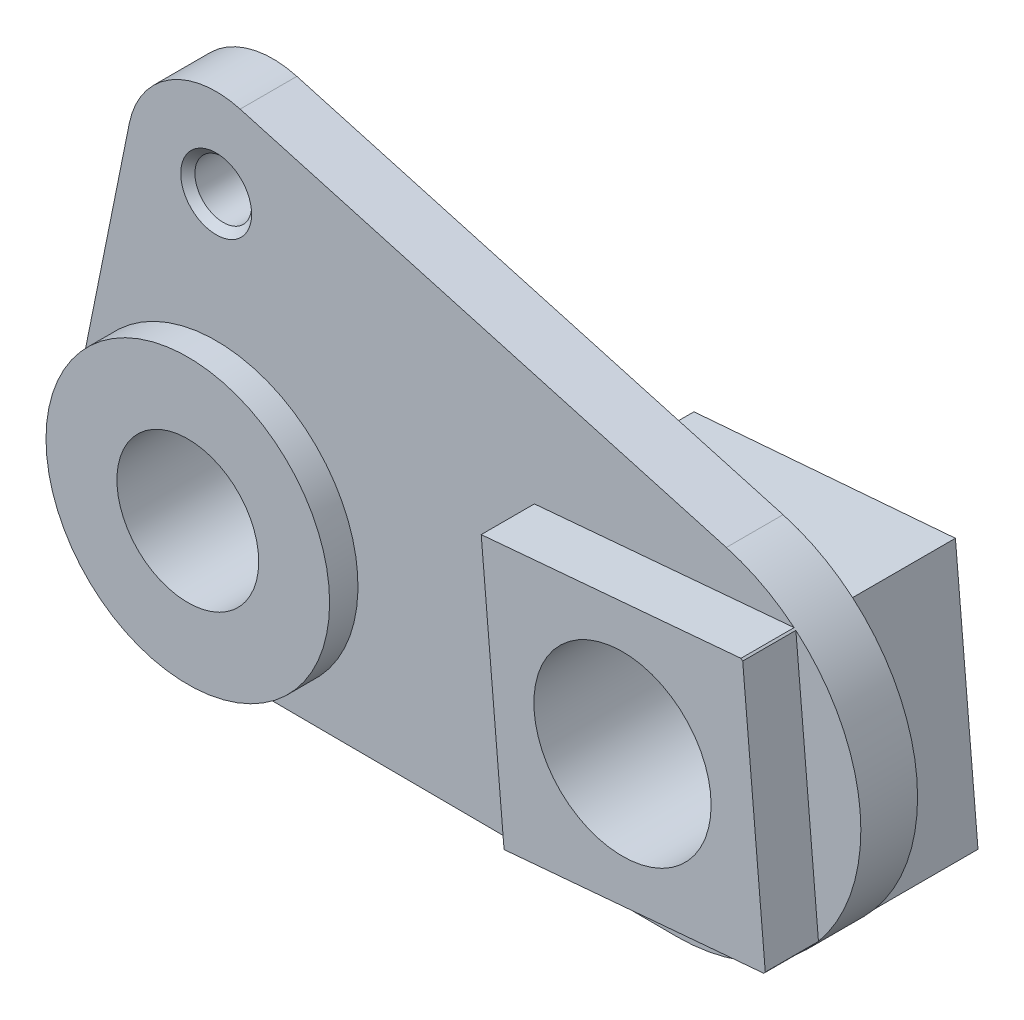
ISO-10303-21;
HEADER;
FILE_DESCRIPTION(('STEP AP214'),'2;1');
FILE_NAME('part.step','',(''),(''),'','','');
FILE_SCHEMA(('AUTOMOTIVE_DESIGN { 1 0 10303 214 1 1 1 1 }'));
ENDSEC;
DATA;
#1=APPLICATION_CONTEXT('core data for automotive mechanical design processes');
#2=APPLICATION_PROTOCOL_DEFINITION('international standard','automotive_design',2000,#1);
#3=PRODUCT_CONTEXT('',#1,'mechanical');
#4=PRODUCT('Part','Part','',(#3));
#5=PRODUCT_RELATED_PRODUCT_CATEGORY('part','',(#4));
#6=PRODUCT_DEFINITION_FORMATION('','',#4);
#7=PRODUCT_DEFINITION_CONTEXT('part definition',#1,'design');
#8=PRODUCT_DEFINITION('design','',#6,#7);
#9=PRODUCT_DEFINITION_SHAPE('','',#8);
#10=(LENGTH_UNIT() NAMED_UNIT(*) SI_UNIT(.MILLI.,.METRE.));
#11=(NAMED_UNIT(*) PLANE_ANGLE_UNIT() SI_UNIT($,.RADIAN.));
#12=(NAMED_UNIT(*) SI_UNIT($,.STERADIAN.) SOLID_ANGLE_UNIT());
#13=UNCERTAINTY_MEASURE_WITH_UNIT(LENGTH_MEASURE(1.E-05),#10,'distance_accuracy_value','');
#14=(GEOMETRIC_REPRESENTATION_CONTEXT(3) GLOBAL_UNCERTAINTY_ASSIGNED_CONTEXT((#13)) GLOBAL_UNIT_ASSIGNED_CONTEXT((#10,
#11,#12)) REPRESENTATION_CONTEXT('',''));
#15=CARTESIAN_POINT('',(0.,0.,0.));
#16=DIRECTION('',(0.,0.,1.));
#17=DIRECTION('',(1.,0.,0.));
#18=AXIS2_PLACEMENT_3D('',#15,#16,#17);
#19=CARTESIAN_POINT('',(0.,0.,0.));
#20=DIRECTION('',(0.,0.,1.));
#21=DIRECTION('',(1.,0.,0.));
#22=AXIS2_PLACEMENT_3D('',#19,#20,#21);
#23=PLANE('',#22);
#24=CARTESIAN_POINT('',(0.,75.86,0.));
#25=DIRECTION('',(0.,0.,1.));
#26=DIRECTION('',(1.,0.,0.));
#27=AXIS2_PLACEMENT_3D('',#24,#25,#26);
#28=CIRCLE('',#27,7.99999999999999);
#29=CARTESIAN_POINT('',(7.99999999999999,75.86,0.));
#30=VERTEX_POINT('',#29);
#31=EDGE_CURVE('E250',#30,#30,#28,.T.);
#32=ORIENTED_EDGE('',*,*,#31,.T.);
#33=EDGE_LOOP('',(#32));
#34=FACE_BOUND('',#33,.T.);
#35=DIRECTION('',(-0.996719788466052,-0.0809299899925204,0.));
#36=VECTOR('',#35,1.);
#37=CARTESIAN_POINT('',(-3.04154501763614,37.4591434753476,0.));
#38=LINE('',#37,#36);
#39=CARTESIAN_POINT('',(163.514258420049,50.9828636436336,0.));
#40=VERTEX_POINT('',#39);
#41=CARTESIAN_POINT('',(89.7555544616044,44.9939274929779,0.));
#42=VERTEX_POINT('',#41);
#43=EDGE_CURVE('E204',#40,#42,#38,.T.);
#44=ORIENTED_EDGE('',*,*,#43,.T.);
#45=DIRECTION('',(0.0871557427476584,-0.996194698091746,0.));
#46=VECTOR('',#45,1.);
#47=CARTESIAN_POINT('',(92.9803169432677,8.13472366358334,0.));
#48=LINE('',#47,#46);
#49=CARTESIAN_POINT('',(96.2050794249311,-28.7244801658113,0.));
#50=VERTEX_POINT('',#49);
#51=EDGE_CURVE('E207',#42,#50,#48,.T.);
#52=ORIENTED_EDGE('',*,*,#51,.T.);
#53=DIRECTION('',(0.99563072054286,0.0933780933158645,0.));
#54=VECTOR('',#53,1.);
#55=CARTESIAN_POINT('',(3.50937488695451,-37.4182136653235,0.));
#56=LINE('',#55,#54);
#57=CARTESIAN_POINT('',(169.883190784065,-21.8143663898134,0.));
#58=VERTEX_POINT('',#57);
#59=EDGE_CURVE('E168',#50,#58,#56,.T.);
#60=ORIENTED_EDGE('',*,*,#59,.T.);
#61=CARTESIAN_POINT('',(129.839520772662,11.3594861452467,0.));
#62=DIRECTION('',(0.,0.,1.));
#63=DIRECTION('',(1.,0.,0.));
#64=AXIS2_PLACEMENT_3D('',#61,#62,#63);
#65=CIRCLE('',#64,52.);
#66=CARTESIAN_POINT('',(129.839520772662,-40.6405138547533,0.));
#67=VERTEX_POINT('',#66);
#68=EDGE_CURVE('E283',#67,#58,#65,.T.);
#69=ORIENTED_EDGE('',*,*,#68,.F.);
#70=DIRECTION('',(0.999987832388727,-0.0049330593444748,0.));
#71=VECTOR('',#70,1.);
#72=CARTESIAN_POINT('',(-0.197319972837052,-39.9990265970202,0.));
#73=LINE('',#72,#71);
#74=CARTESIAN_POINT('',(0.,-40.,0.));
#75=VERTEX_POINT('',#74);
#76=EDGE_CURVE('E259',#75,#67,#73,.T.);
#77=ORIENTED_EDGE('',*,*,#76,.F.);
#78=CARTESIAN_POINT('',(0.,0.,0.));
#79=DIRECTION('',(0.,0.,-1.));
#80=DIRECTION('',(-1.,0.,0.));
#81=AXIS2_PLACEMENT_3D('',#78,#79,#80);
#82=CIRCLE('',#81,40.);
#83=CARTESIAN_POINT('',(-39.2102393365701,7.9093066174532,0.));
#84=VERTEX_POINT('',#83);
#85=EDGE_CURVE('E249',#84,#75,#82,.T.);
#86=ORIENTED_EDGE('',*,*,#85,.F.);
#87=DIRECTION('',(-0.19773266543633,-0.980255983414253,0.));
#88=VECTOR('',#87,1.);
#89=CARTESIAN_POINT('',(-39.2102393365701,7.90930661745321,0.));
#90=LINE('',#89,#88);
#91=CARTESIAN_POINT('',(-24.5063995853563,80.8033166359082,0.));
#92=VERTEX_POINT('',#91);
#93=EDGE_CURVE('E270',#92,#84,#90,.T.);
#94=ORIENTED_EDGE('',*,*,#93,.F.);
#95=CARTESIAN_POINT('',(0.,75.86,0.));
#96=DIRECTION('',(0.,0.,1.));
#97=DIRECTION('',(1.,0.,0.));
#98=AXIS2_PLACEMENT_3D('',#95,#96,#97);
#99=CIRCLE('',#98,25.);
#100=CARTESIAN_POINT('',(6.75816471696034,99.9292170553683,0.));
#101=VERTEX_POINT('',#100);
#102=EDGE_CURVE('E288',#101,#92,#99,.T.);
#103=ORIENTED_EDGE('',*,*,#102,.F.);
#104=DIRECTION('',(0.962768682214732,-0.270326588678414,0.));
#105=VECTOR('',#104,1.);
#106=CARTESIAN_POINT('',(26.5016380304269,94.3856364548702,0.));
#107=LINE('',#106,#105);
#108=CARTESIAN_POINT('',(143.89650338394,61.4234576204128,0.));
#109=VERTEX_POINT('',#108);
#110=EDGE_CURVE('E287',#101,#109,#107,.T.);
#111=ORIENTED_EDGE('',*,*,#110,.T.);
#112=EDGE_CURVE('E285',#40,#109,#65,.T.);
#113=ORIENTED_EDGE('',*,*,#112,.F.);
#114=EDGE_LOOP('',(#44,#52,#60,#69,#77,#86,#94,#103,#111,#113));
#115=FACE_BOUND('',#114,.T.);
#116=ADVANCED_FACE('F47',(#34,#115),#23,.F.);
#117=CARTESIAN_POINT('',(0.,0.,16.));
#118=DIRECTION('',(0.,0.,1.));
#119=DIRECTION('',(1.,0.,0.));
#120=AXIS2_PLACEMENT_3D('',#117,#118,#119);
#121=PLANE('',#120);
#122=DIRECTION('',(0.996194698091746,0.0871557427476586,0.));
#123=VECTOR('',#122,1.);
#124=CARTESIAN_POINT('',(-3.22476248166336,36.8592038293946,16.));
#125=LINE('',#124,#123);
#126=CARTESIAN_POINT('',(89.7555544616044,44.9939274929779,16.));
#127=VERTEX_POINT('',#126);
#128=CARTESIAN_POINT('',(163.013373307722,51.4031561566491,16.));
#129=VERTEX_POINT('',#128);
#130=EDGE_CURVE('E206',#127,#129,#125,.T.);
#131=ORIENTED_EDGE('',*,*,#130,.T.);
#132=CARTESIAN_POINT('',(129.839520772662,11.3594861452467,16.));
#133=DIRECTION('',(0.,0.,1.));
#134=DIRECTION('',(1.,0.,0.));
#135=AXIS2_PLACEMENT_3D('',#132,#133,#134);
#136=CIRCLE('',#135,52.);
#137=CARTESIAN_POINT('',(143.89650338394,61.4234576204128,16.));
#138=VERTEX_POINT('',#137);
#139=EDGE_CURVE('E267',#129,#138,#136,.T.);
#140=ORIENTED_EDGE('',*,*,#139,.T.);
#141=DIRECTION('',(0.962768682214732,-0.270326588678414,0.));
#142=VECTOR('',#141,1.);
#143=CARTESIAN_POINT('',(26.5016380304269,94.3856364548702,16.));
#144=LINE('',#143,#142);
#145=CARTESIAN_POINT('',(6.75816471696034,99.9292170553683,16.));
#146=VERTEX_POINT('',#145);
#147=EDGE_CURVE('E268',#146,#138,#144,.T.);
#148=ORIENTED_EDGE('',*,*,#147,.F.);
#149=CARTESIAN_POINT('',(0.,75.86,16.));
#150=DIRECTION('',(0.,0.,1.));
#151=DIRECTION('',(1.,0.,0.));
#152=AXIS2_PLACEMENT_3D('',#149,#150,#151);
#153=CIRCLE('',#152,25.);
#154=CARTESIAN_POINT('',(-24.5063995853563,80.8033166359082,16.));
#155=VERTEX_POINT('',#154);
#156=EDGE_CURVE('E274',#146,#155,#153,.T.);
#157=ORIENTED_EDGE('',*,*,#156,.T.);
#158=DIRECTION('',(-0.19773266543633,-0.980255983414253,0.));
#159=VECTOR('',#158,1.);
#160=CARTESIAN_POINT('',(-39.2102393365701,7.90930661745321,16.));
#161=LINE('',#160,#159);
#162=CARTESIAN_POINT('',(-39.2102393365701,7.9093066174532,16.));
#163=VERTEX_POINT('',#162);
#164=EDGE_CURVE('E277',#155,#163,#161,.T.);
#165=ORIENTED_EDGE('',*,*,#164,.T.);
#166=CARTESIAN_POINT('',(0.,0.,16.));
#167=DIRECTION('',(0.,0.,1.));
#168=DIRECTION('',(1.,0.,0.));
#169=AXIS2_PLACEMENT_3D('',#166,#167,#168);
#170=CIRCLE('',#169,40.);
#171=CARTESIAN_POINT('',(0.,-40.,16.));
#172=VERTEX_POINT('',#171);
#173=EDGE_CURVE('E256',#172,#163,#170,.T.);
#174=ORIENTED_EDGE('',*,*,#173,.F.);
#175=DIRECTION('',(0.999987832388727,-0.0049330593444748,0.));
#176=VECTOR('',#175,1.);
#177=CARTESIAN_POINT('',(-0.197319972837052,-39.9990265970202,16.));
#178=LINE('',#177,#176);
#179=CARTESIAN_POINT('',(129.839520772662,-40.6405138547533,16.));
#180=VERTEX_POINT('',#179);
#181=EDGE_CURVE('E263',#172,#180,#178,.T.);
#182=ORIENTED_EDGE('',*,*,#181,.T.);
#183=CARTESIAN_POINT('',(169.462898271049,-22.3152515021401,16.));
#184=VERTEX_POINT('',#183);
#185=EDGE_CURVE('E269',#180,#184,#136,.T.);
#186=ORIENTED_EDGE('',*,*,#185,.T.);
#187=DIRECTION('',(-0.996194698091746,-0.0871557427476586,0.));
#188=VECTOR('',#187,1.);
#189=CARTESIAN_POINT('',(3.22476248166337,-36.8592038293946,16.));
#190=LINE('',#189,#188);
#191=CARTESIAN_POINT('',(96.2050794249311,-28.7244801658113,16.));
#192=VERTEX_POINT('',#191);
#193=EDGE_CURVE('E226',#184,#192,#190,.T.);
#194=ORIENTED_EDGE('',*,*,#193,.T.);
#195=DIRECTION('',(-0.0871557427476586,0.996194698091746,0.));
#196=VECTOR('',#195,1.);
#197=CARTESIAN_POINT('',(92.9803169432677,8.13472366358337,16.));
#198=LINE('',#197,#196);
#199=EDGE_CURVE('E74',#192,#127,#198,.T.);
#200=ORIENTED_EDGE('',*,*,#199,.T.);
#201=EDGE_LOOP('',(#131,#140,#148,#157,#165,#174,#182,#186,#194,#200));
#202=FACE_BOUND('',#201,.T.);
#203=CARTESIAN_POINT('',(0.,75.86,16.));
#204=DIRECTION('',(0.,0.,1.));
#205=DIRECTION('',(1.,0.,0.));
#206=AXIS2_PLACEMENT_3D('',#203,#204,#205);
#207=CIRCLE('',#206,9.99999999999998);
#208=CARTESIAN_POINT('',(9.99999999999998,75.86,16.));
#209=VERTEX_POINT('',#208);
#210=EDGE_CURVE('E11',#209,#209,#207,.F.);
#211=ORIENTED_EDGE('',*,*,#210,.T.);
#212=EDGE_LOOP('',(#211));
#213=FACE_BOUND('',#212,.T.);
#214=ADVANCED_FACE('F328',(#202,#213),#121,.T.);
#215=EDGE_CURVE('E290',#58,#40,#65,.T.);
#216=ORIENTED_EDGE('',*,*,#215,.F.);
#217=DIRECTION('',(-0.0871557427476589,0.996194698091746,0.));
#218=VECTOR('',#217,1.);
#219=CARTESIAN_POINT('',(166.698724602057,14.5842486269101,0.));
#220=LINE('',#219,#218);
#221=EDGE_CURVE('E199',#58,#40,#220,.T.);
#222=ORIENTED_EDGE('',*,*,#221,.T.);
#223=EDGE_LOOP('',(#216,#222));
#224=FACE_BOUND('',#223,.T.);
#225=ADVANCED_FACE('F332',(#224),#23,.F.);
#226=CARTESIAN_POINT('',(-0.197319972837052,-39.9990265970202,16.));
#227=DIRECTION('',(0.0049330593444748,0.999987832388726,0.));
#228=DIRECTION('',(-0.999987832388727,0.0049330593444748,0.));
#229=AXIS2_PLACEMENT_3D('',#226,#227,#228);
#230=PLANE('',#229);
#231=ORIENTED_EDGE('',*,*,#76,.T.);
#232=DIRECTION('',(0.,0.,-1.));
#233=VECTOR('',#232,1.);
#234=CARTESIAN_POINT('',(129.839520772662,-40.6405138547533,16.));
#235=LINE('',#234,#233);
#236=EDGE_CURVE('E265',#180,#67,#235,.T.);
#237=ORIENTED_EDGE('',*,*,#236,.F.);
#238=ORIENTED_EDGE('',*,*,#181,.F.);
#239=DIRECTION('',(0.,0.,-1.));
#240=VECTOR('',#239,1.);
#241=CARTESIAN_POINT('',(0.,-40.,16.));
#242=LINE('',#241,#240);
#243=EDGE_CURVE('E276',#172,#75,#242,.T.);
#244=ORIENTED_EDGE('',*,*,#243,.T.);
#245=EDGE_LOOP('',(#231,#237,#238,#244));
#246=FACE_BOUND('',#245,.T.);
#247=ADVANCED_FACE('F342',(#246),#230,.F.);
#248=CARTESIAN_POINT('',(129.839520772662,11.3594861452467,16.));
#249=DIRECTION('',(0.,0.,-1.));
#250=DIRECTION('',(-1.,0.,0.));
#251=AXIS2_PLACEMENT_3D('',#248,#249,#250);
#252=CYLINDRICAL_SURFACE('',#251,52.);
#253=ORIENTED_EDGE('',*,*,#68,.T.);
#254=ORIENTED_EDGE('',*,*,#215,.T.);
#255=ORIENTED_EDGE('',*,*,#112,.T.);
#256=DIRECTION('',(0.,0.,-1.));
#257=VECTOR('',#256,1.);
#258=CARTESIAN_POINT('',(143.89650338394,61.4234576204128,16.));
#259=LINE('',#258,#257);
#260=EDGE_CURVE('E302',#138,#109,#259,.T.);
#261=ORIENTED_EDGE('',*,*,#260,.F.);
#262=ORIENTED_EDGE('',*,*,#139,.F.);
#263=DIRECTION('',(0.,0.,-1.));
#264=VECTOR('',#263,1.);
#265=CARTESIAN_POINT('',(163.013373307722,51.4031561566491,31.));
#266=LINE('',#265,#264);
#267=CARTESIAN_POINT('',(163.013373307722,51.4031561566491,31.));
#268=VERTEX_POINT('',#267);
#269=EDGE_CURVE('E242',#268,#129,#266,.T.);
#270=ORIENTED_EDGE('',*,*,#269,.F.);
#271=CARTESIAN_POINT('',(129.839520772662,11.3594861452467,31.));
#272=DIRECTION('',(0.,0.,1.));
#273=DIRECTION('',(1.,0.,0.));
#274=AXIS2_PLACEMENT_3D('',#271,#272,#273);
#275=CIRCLE('',#274,52.);
#276=CARTESIAN_POINT('',(163.514258420049,50.9828636436336,31.));
#277=VERTEX_POINT('',#276);
#278=EDGE_CURVE('E209',#277,#268,#275,.T.);
#279=ORIENTED_EDGE('',*,*,#278,.F.);
#280=DIRECTION('',(0.,0.,-1.));
#281=VECTOR('',#280,1.);
#282=CARTESIAN_POINT('',(163.514258420049,50.9828636436336,31.));
#283=LINE('',#282,#281);
#284=CARTESIAN_POINT('',(163.514258420049,50.9828636436336,16.));
#285=VERTEX_POINT('',#284);
#286=EDGE_CURVE('E223',#277,#285,#283,.T.);
#287=ORIENTED_EDGE('',*,*,#286,.T.);
#288=CARTESIAN_POINT('',(169.883190784065,-21.8143663898134,16.));
#289=VERTEX_POINT('',#288);
#290=EDGE_CURVE('E272',#289,#285,#136,.T.);
#291=ORIENTED_EDGE('',*,*,#290,.F.);
#292=DIRECTION('',(0.,0.,-1.));
#293=VECTOR('',#292,1.);
#294=CARTESIAN_POINT('',(169.883190784065,-21.8143663898134,31.));
#295=LINE('',#294,#293);
#296=CARTESIAN_POINT('',(169.883190784065,-21.8143663898134,31.));
#297=VERTEX_POINT('',#296);
#298=EDGE_CURVE('E231',#297,#289,#295,.T.);
#299=ORIENTED_EDGE('',*,*,#298,.F.);
#300=CARTESIAN_POINT('',(169.462898271049,-22.3152515021401,31.));
#301=VERTEX_POINT('',#300);
#302=EDGE_CURVE('E214',#301,#297,#275,.T.);
#303=ORIENTED_EDGE('',*,*,#302,.F.);
#304=DIRECTION('',(0.,0.,-1.));
#305=VECTOR('',#304,1.);
#306=CARTESIAN_POINT('',(169.462898271049,-22.3152515021401,31.));
#307=LINE('',#306,#305);
#308=EDGE_CURVE('E236',#301,#184,#307,.T.);
#309=ORIENTED_EDGE('',*,*,#308,.T.);
#310=ORIENTED_EDGE('',*,*,#185,.F.);
#311=ORIENTED_EDGE('',*,*,#236,.T.);
#312=EDGE_LOOP('',(#253,#254,#255,#261,#262,#270,#279,#287,#291,#299,#303,#309,#310,#311));
#313=FACE_BOUND('',#312,.T.);
#314=ADVANCED_FACE('F350',(#313),#252,.T.);
#315=CARTESIAN_POINT('',(26.5016380304269,94.3856364548702,16.));
#316=DIRECTION('',(0.270326588678414,0.962768682214732,0.));
#317=DIRECTION('',(-0.962768682214732,0.270326588678414,0.));
#318=AXIS2_PLACEMENT_3D('',#315,#316,#317);
#319=PLANE('',#318);
#320=ORIENTED_EDGE('',*,*,#110,.F.);
#321=DIRECTION('',(0.,0.,-1.));
#322=VECTOR('',#321,1.);
#323=CARTESIAN_POINT('',(6.75816471696034,99.9292170553683,16.));
#324=LINE('',#323,#322);
#325=EDGE_CURVE('E305',#146,#101,#324,.T.);
#326=ORIENTED_EDGE('',*,*,#325,.F.);
#327=ORIENTED_EDGE('',*,*,#147,.T.);
#328=ORIENTED_EDGE('',*,*,#260,.T.);
#329=EDGE_LOOP('',(#320,#326,#327,#328));
#330=FACE_BOUND('',#329,.T.);
#331=ADVANCED_FACE('F426',(#330),#319,.T.);
#332=CARTESIAN_POINT('',(0.,75.86,16.));
#333=DIRECTION('',(0.,0.,-1.));
#334=DIRECTION('',(-1.,0.,0.));
#335=AXIS2_PLACEMENT_3D('',#332,#333,#334);
#336=CYLINDRICAL_SURFACE('',#335,25.);
#337=ORIENTED_EDGE('',*,*,#102,.T.);
#338=DIRECTION('',(0.,0.,-1.));
#339=VECTOR('',#338,1.);
#340=CARTESIAN_POINT('',(-24.5063995853563,80.8033166359082,16.));
#341=LINE('',#340,#339);
#342=EDGE_CURVE('E299',#155,#92,#341,.T.);
#343=ORIENTED_EDGE('',*,*,#342,.F.);
#344=ORIENTED_EDGE('',*,*,#156,.F.);
#345=ORIENTED_EDGE('',*,*,#325,.T.);
#346=EDGE_LOOP('',(#337,#343,#344,#345));
#347=FACE_BOUND('',#346,.T.);
#348=ADVANCED_FACE('F425',(#347),#336,.T.);
#349=CARTESIAN_POINT('',(-39.2102393365701,7.90930661745321,16.));
#350=DIRECTION('',(0.980255983414253,-0.19773266543633,0.));
#351=DIRECTION('',(0.19773266543633,0.980255983414253,0.));
#352=AXIS2_PLACEMENT_3D('',#349,#350,#351);
#353=PLANE('',#352);
#354=ORIENTED_EDGE('',*,*,#93,.T.);
#355=DIRECTION('',(0.,0.,-1.));
#356=VECTOR('',#355,1.);
#357=CARTESIAN_POINT('',(-39.2102393365701,7.90930661745321,16.));
#358=LINE('',#357,#356);
#359=EDGE_CURVE('E298',#163,#84,#358,.T.);
#360=ORIENTED_EDGE('',*,*,#359,.F.);
#361=ORIENTED_EDGE('',*,*,#164,.F.);
#362=ORIENTED_EDGE('',*,*,#342,.T.);
#363=EDGE_LOOP('',(#354,#360,#361,#362));
#364=FACE_BOUND('',#363,.T.);
#365=ADVANCED_FACE('F396',(#364),#353,.F.);
#366=CARTESIAN_POINT('',(0.,0.,16.));
#367=DIRECTION('',(0.,0.,-1.));
#368=DIRECTION('',(-1.,0.,0.));
#369=AXIS2_PLACEMENT_3D('',#366,#367,#368);
#370=CYLINDRICAL_SURFACE('',#369,40.);
#371=ORIENTED_EDGE('',*,*,#359,.T.);
#372=ORIENTED_EDGE('',*,*,#85,.T.);
#373=ORIENTED_EDGE('',*,*,#243,.F.);
#374=ORIENTED_EDGE('',*,*,#173,.T.);
#375=EDGE_LOOP('',(#371,#372,#373,#374));
#376=FACE_BOUND('',#375,.T.);
#377=CARTESIAN_POINT('',(0.,0.,24.));
#378=DIRECTION('',(0.,0.,1.));
#379=DIRECTION('',(1.,0.,0.));
#380=AXIS2_PLACEMENT_3D('',#377,#378,#379);
#381=CIRCLE('',#380,40.);
#382=CARTESIAN_POINT('',(40.,0.,24.));
#383=VERTEX_POINT('',#382);
#384=EDGE_CURVE('E251',#383,#383,#381,.T.);
#385=ORIENTED_EDGE('',*,*,#384,.F.);
#386=EDGE_LOOP('',(#385));
#387=FACE_BOUND('',#386,.T.);
#388=CARTESIAN_POINT('',(0.,0.,-16.));
#389=DIRECTION('',(0.,0.,-1.));
#390=DIRECTION('',(-1.,0.,0.));
#391=AXIS2_PLACEMENT_3D('',#388,#389,#390);
#392=CIRCLE('',#391,40.);
#393=CARTESIAN_POINT('',(-40.,0.,-16.));
#394=VERTEX_POINT('',#393);
#395=EDGE_CURVE('E252',#394,#394,#392,.T.);
#396=ORIENTED_EDGE('',*,*,#395,.F.);
#397=EDGE_LOOP('',(#396));
#398=FACE_BOUND('',#397,.T.);
#399=ADVANCED_FACE('F393',(#376,#387,#398),#370,.T.);
#400=DIRECTION('',(0.0871557427476586,-0.996194698091746,0.));
#401=VECTOR('',#400,1.);
#402=CARTESIAN_POINT('',(166.698724602057,14.5842486269101,16.));
#403=LINE('',#402,#401);
#404=EDGE_CURVE('E215',#285,#289,#403,.T.);
#405=ORIENTED_EDGE('',*,*,#404,.T.);
#406=ORIENTED_EDGE('',*,*,#290,.T.);
#407=EDGE_LOOP('',(#405,#406));
#408=FACE_BOUND('',#407,.T.);
#409=ADVANCED_FACE('F336',(#408),#121,.T.);
#410=CARTESIAN_POINT('',(0.,0.,24.));
#411=DIRECTION('',(0.,0.,1.));
#412=DIRECTION('',(1.,0.,0.));
#413=AXIS2_PLACEMENT_3D('',#410,#411,#412);
#414=PLANE('',#413);
#415=CARTESIAN_POINT('',(0.,0.,24.));
#416=DIRECTION('',(0.,0.,1.));
#417=DIRECTION('',(1.,0.,0.));
#418=AXIS2_PLACEMENT_3D('',#415,#416,#417);
#419=CIRCLE('',#418,20.);
#420=CARTESIAN_POINT('',(20.,0.,24.));
#421=VERTEX_POINT('',#420);
#422=EDGE_CURVE('E715',#421,#421,#419,.T.);
#423=ORIENTED_EDGE('',*,*,#422,.F.);
#424=EDGE_LOOP('',(#423));
#425=FACE_BOUND('',#424,.T.);
#426=ORIENTED_EDGE('',*,*,#384,.T.);
#427=EDGE_LOOP('',(#426));
#428=FACE_BOUND('',#427,.T.);
#429=ADVANCED_FACE('F389',(#425,#428),#414,.T.);
#430=CARTESIAN_POINT('',(0.,0.,-16.));
#431=DIRECTION('',(0.,0.,-1.));
#432=DIRECTION('',(-1.,0.,0.));
#433=AXIS2_PLACEMENT_3D('',#430,#431,#432);
#434=PLANE('',#433);
#435=CARTESIAN_POINT('',(0.,0.,-16.));
#436=DIRECTION('',(0.,0.,1.));
#437=DIRECTION('',(1.,0.,0.));
#438=AXIS2_PLACEMENT_3D('',#435,#436,#437);
#439=CIRCLE('',#438,20.);
#440=CARTESIAN_POINT('',(20.,0.,-16.));
#441=VERTEX_POINT('',#440);
#442=EDGE_CURVE('E706',#441,#441,#439,.T.);
#443=ORIENTED_EDGE('',*,*,#442,.T.);
#444=EDGE_LOOP('',(#443));
#445=FACE_BOUND('',#444,.T.);
#446=ORIENTED_EDGE('',*,*,#395,.T.);
#447=EDGE_LOOP('',(#446));
#448=FACE_BOUND('',#447,.T.);
#449=ADVANCED_FACE('F321',(#445,#448),#434,.T.);
#450=CARTESIAN_POINT('',(0.,75.86,0.));
#451=DIRECTION('',(0.,0.,1.));
#452=DIRECTION('',(1.,0.,0.));
#453=AXIS2_PLACEMENT_3D('',#450,#451,#452);
#454=CYLINDRICAL_SURFACE('',#453,7.99999999999999);
#455=CARTESIAN_POINT('',(0.,75.86,14.));
#456=DIRECTION('',(0.,0.,1.));
#457=DIRECTION('',(1.,0.,0.));
#458=AXIS2_PLACEMENT_3D('',#455,#456,#457);
#459=CIRCLE('',#458,7.99999999999999);
#460=CARTESIAN_POINT('',(7.99999999999999,75.86,14.));
#461=VERTEX_POINT('',#460);
#462=EDGE_CURVE('E59',#461,#461,#459,.T.);
#463=ORIENTED_EDGE('',*,*,#462,.T.);
#464=EDGE_LOOP('',(#463));
#465=FACE_BOUND('',#464,.T.);
#466=ORIENTED_EDGE('',*,*,#31,.F.);
#467=EDGE_LOOP('',(#466));
#468=FACE_BOUND('',#467,.T.);
#469=ADVANCED_FACE('F311',(#465,#468),#454,.F.);
#470=CARTESIAN_POINT('',(0.,75.86,14.));
#471=DIRECTION('',(0.,0.,1.));
#472=DIRECTION('',(1.,0.,0.));
#473=AXIS2_PLACEMENT_3D('',#470,#471,#472);
#474=CONICAL_SURFACE('',#473,7.99999999999999,0.785398163397448);
#475=ORIENTED_EDGE('',*,*,#210,.F.);
#476=EDGE_LOOP('',(#475));
#477=FACE_BOUND('',#476,.T.);
#478=ORIENTED_EDGE('',*,*,#462,.F.);
#479=EDGE_LOOP('',(#478));
#480=FACE_BOUND('',#479,.T.);
#481=ADVANCED_FACE('F55',(#477,#480),#474,.F.);
#482=CARTESIAN_POINT('',(-3.22476248166336,36.8592038293946,31.));
#483=DIRECTION('',(-0.0871557427476586,0.996194698091746,0.));
#484=DIRECTION('',(-0.996194698091746,-0.0871557427476586,0.));
#485=AXIS2_PLACEMENT_3D('',#482,#483,#484);
#486=PLANE('',#485);
#487=ORIENTED_EDGE('',*,*,#130,.F.);
#488=DIRECTION('',(0.,0.,-1.));
#489=VECTOR('',#488,1.);
#490=CARTESIAN_POINT('',(89.7555544616044,44.9939274929779,31.));
#491=LINE('',#490,#489);
#492=CARTESIAN_POINT('',(89.7555544616044,44.9939274929779,31.));
#493=VERTEX_POINT('',#492);
#494=EDGE_CURVE('E245',#493,#127,#491,.T.);
#495=ORIENTED_EDGE('',*,*,#494,.F.);
#496=DIRECTION('',(0.996194698091746,0.0871557427476586,0.));
#497=VECTOR('',#496,1.);
#498=CARTESIAN_POINT('',(-3.22476248166336,36.8592038293946,31.));
#499=LINE('',#498,#497);
#500=EDGE_CURVE('E212',#493,#268,#499,.T.);
#501=ORIENTED_EDGE('',*,*,#500,.T.);
#502=ORIENTED_EDGE('',*,*,#269,.T.);
#503=EDGE_LOOP('',(#487,#495,#501,#502));
#504=FACE_BOUND('',#503,.T.);
#505=ADVANCED_FACE('F314',(#504),#486,.T.);
#506=CARTESIAN_POINT('',(92.9803169432677,8.13472366358337,31.));
#507=DIRECTION('',(-0.996194698091746,-0.0871557427476586,0.));
#508=DIRECTION('',(0.0871557427476586,-0.996194698091746,0.));
#509=AXIS2_PLACEMENT_3D('',#506,#507,#508);
#510=PLANE('',#509);
#511=ORIENTED_EDGE('',*,*,#199,.F.);
#512=DIRECTION('',(0.,0.,-1.));
#513=VECTOR('',#512,1.);
#514=CARTESIAN_POINT('',(96.2050794249311,-28.7244801658113,31.));
#515=LINE('',#514,#513);
#516=CARTESIAN_POINT('',(96.2050794249311,-28.7244801658113,31.));
#517=VERTEX_POINT('',#516);
#518=EDGE_CURVE('E237',#517,#192,#515,.T.);
#519=ORIENTED_EDGE('',*,*,#518,.F.);
#520=DIRECTION('',(-0.0871557427476586,0.996194698091746,0.));
#521=VECTOR('',#520,1.);
#522=CARTESIAN_POINT('',(92.9803169432677,8.13472366358337,31.));
#523=LINE('',#522,#521);
#524=EDGE_CURVE('E216',#517,#493,#523,.T.);
#525=ORIENTED_EDGE('',*,*,#524,.T.);
#526=ORIENTED_EDGE('',*,*,#494,.T.);
#527=EDGE_LOOP('',(#511,#519,#525,#526));
#528=FACE_BOUND('',#527,.T.);
#529=ADVANCED_FACE('F322',(#528),#510,.T.);
#530=CARTESIAN_POINT('',(3.22476248166337,-36.8592038293946,31.));
#531=DIRECTION('',(0.0871557427476586,-0.996194698091746,0.));
#532=DIRECTION('',(0.996194698091746,0.0871557427476586,0.));
#533=AXIS2_PLACEMENT_3D('',#530,#531,#532);
#534=PLANE('',#533);
#535=ORIENTED_EDGE('',*,*,#193,.F.);
#536=ORIENTED_EDGE('',*,*,#308,.F.);
#537=DIRECTION('',(-0.996194698091746,-0.0871557427476586,0.));
#538=VECTOR('',#537,1.);
#539=CARTESIAN_POINT('',(3.22476248166337,-36.8592038293946,31.));
#540=LINE('',#539,#538);
#541=EDGE_CURVE('E217',#301,#517,#540,.T.);
#542=ORIENTED_EDGE('',*,*,#541,.T.);
#543=ORIENTED_EDGE('',*,*,#518,.T.);
#544=EDGE_LOOP('',(#535,#536,#542,#543));
#545=FACE_BOUND('',#544,.T.);
#546=ADVANCED_FACE('F377',(#545),#534,.T.);
#547=CARTESIAN_POINT('',(166.698724602057,14.5842486269101,31.));
#548=DIRECTION('',(0.996194698091746,0.0871557427476586,0.));
#549=DIRECTION('',(-0.0871557427476586,0.996194698091746,0.));
#550=AXIS2_PLACEMENT_3D('',#547,#548,#549);
#551=PLANE('',#550);
#552=ORIENTED_EDGE('',*,*,#404,.F.);
#553=ORIENTED_EDGE('',*,*,#286,.F.);
#554=DIRECTION('',(0.0871557427476586,-0.996194698091746,0.));
#555=VECTOR('',#554,1.);
#556=CARTESIAN_POINT('',(166.698724602057,14.5842486269101,31.));
#557=LINE('',#556,#555);
#558=EDGE_CURVE('E225',#277,#297,#557,.T.);
#559=ORIENTED_EDGE('',*,*,#558,.T.);
#560=ORIENTED_EDGE('',*,*,#298,.T.);
#561=EDGE_LOOP('',(#552,#553,#559,#560));
#562=FACE_BOUND('',#561,.T.);
#563=ADVANCED_FACE('F372',(#562),#551,.T.);
#564=CARTESIAN_POINT('',(0.,0.,31.));
#565=DIRECTION('',(0.,0.,1.));
#566=DIRECTION('',(1.,0.,0.));
#567=AXIS2_PLACEMENT_3D('',#564,#565,#566);
#568=PLANE('',#567);
#569=CARTESIAN_POINT('',(129.609226366327,11.3393379954189,31.));
#570=DIRECTION('',(0.,0.,1.));
#571=DIRECTION('',(1.,0.,0.));
#572=AXIS2_PLACEMENT_3D('',#569,#570,#571);
#573=CIRCLE('',#572,25.);
#574=CARTESIAN_POINT('',(154.609226366327,11.3393379954189,31.));
#575=VERTEX_POINT('',#574);
#576=EDGE_CURVE('E189',#575,#575,#573,.T.);
#577=ORIENTED_EDGE('',*,*,#576,.F.);
#578=EDGE_LOOP('',(#577));
#579=FACE_BOUND('',#578,.T.);
#580=ORIENTED_EDGE('',*,*,#302,.T.);
#581=ORIENTED_EDGE('',*,*,#558,.F.);
#582=ORIENTED_EDGE('',*,*,#278,.T.);
#583=ORIENTED_EDGE('',*,*,#500,.F.);
#584=ORIENTED_EDGE('',*,*,#524,.F.);
#585=ORIENTED_EDGE('',*,*,#541,.F.);
#586=EDGE_LOOP('',(#580,#581,#582,#583,#584,#585));
#587=FACE_BOUND('',#586,.T.);
#588=ADVANCED_FACE('F371',(#579,#587),#568,.T.);
#589=CARTESIAN_POINT('',(89.7555544616044,44.9939274929779,-29.));
#590=DIRECTION('',(-0.996194698091746,-0.0871557427476584,0.));
#591=DIRECTION('',(0.0871557427476584,-0.996194698091746,0.));
#592=AXIS2_PLACEMENT_3D('',#589,#590,#591);
#593=PLANE('',#592);
#594=ORIENTED_EDGE('',*,*,#51,.F.);
#595=DIRECTION('',(0.,0.,1.));
#596=VECTOR('',#595,1.);
#597=CARTESIAN_POINT('',(89.7555544616044,44.9939274929779,-29.));
#598=LINE('',#597,#596);
#599=CARTESIAN_POINT('',(89.7555544616044,44.9939274929779,-29.));
#600=VERTEX_POINT('',#599);
#601=EDGE_CURVE('E183',#600,#42,#598,.T.);
#602=ORIENTED_EDGE('',*,*,#601,.F.);
#603=DIRECTION('',(0.0871557427476584,-0.996194698091745,0.));
#604=VECTOR('',#603,1.);
#605=CARTESIAN_POINT('',(89.7555544616044,44.9939274929779,-29.));
#606=LINE('',#605,#604);
#607=CARTESIAN_POINT('',(96.2050794249311,-28.7244801658113,-29.));
#608=VERTEX_POINT('',#607);
#609=EDGE_CURVE('E180',#600,#608,#606,.T.);
#610=ORIENTED_EDGE('',*,*,#609,.T.);
#611=DIRECTION('',(0.,0.,1.));
#612=VECTOR('',#611,1.);
#613=CARTESIAN_POINT('',(96.2050794249311,-28.7244801658113,-29.));
#614=LINE('',#613,#612);
#615=EDGE_CURVE('E163',#608,#50,#614,.T.);
#616=ORIENTED_EDGE('',*,*,#615,.T.);
#617=EDGE_LOOP('',(#594,#602,#610,#616));
#618=FACE_BOUND('',#617,.T.);
#619=ADVANCED_FACE('F185',(#618),#593,.T.);
#620=CARTESIAN_POINT('',(89.7555544616044,44.9939274929779,-29.));
#621=DIRECTION('',(-0.0809299899925204,0.996719788466052,0.));
#622=DIRECTION('',(-0.996719788466052,-0.0809299899925204,0.));
#623=AXIS2_PLACEMENT_3D('',#620,#621,#622);
#624=PLANE('',#623);
#625=ORIENTED_EDGE('',*,*,#43,.F.);
#626=DIRECTION('',(0.,0.,1.));
#627=VECTOR('',#626,1.);
#628=CARTESIAN_POINT('',(163.514258420049,50.9828636436336,-29.));
#629=LINE('',#628,#627);
#630=CARTESIAN_POINT('',(163.514258420049,50.9828636436336,-29.));
#631=VERTEX_POINT('',#630);
#632=EDGE_CURVE('E193',#631,#40,#629,.T.);
#633=ORIENTED_EDGE('',*,*,#632,.F.);
#634=DIRECTION('',(-0.996719788466052,-0.0809299899925204,0.));
#635=VECTOR('',#634,1.);
#636=CARTESIAN_POINT('',(89.7555544616044,44.9939274929779,-29.));
#637=LINE('',#636,#635);
#638=EDGE_CURVE('E167',#631,#600,#637,.T.);
#639=ORIENTED_EDGE('',*,*,#638,.T.);
#640=ORIENTED_EDGE('',*,*,#601,.T.);
#641=EDGE_LOOP('',(#625,#633,#639,#640));
#642=FACE_BOUND('',#641,.T.);
#643=ADVANCED_FACE('F358',(#642),#624,.T.);
#644=CARTESIAN_POINT('',(169.883190784065,-21.8143663898134,-29.));
#645=DIRECTION('',(0.996194698091746,0.0871557427476589,0.));
#646=DIRECTION('',(-0.0871557427476589,0.996194698091746,0.));
#647=AXIS2_PLACEMENT_3D('',#644,#645,#646);
#648=PLANE('',#647);
#649=ORIENTED_EDGE('',*,*,#221,.F.);
#650=DIRECTION('',(0.,0.,1.));
#651=VECTOR('',#650,1.);
#652=CARTESIAN_POINT('',(169.883190784065,-21.8143663898134,-29.));
#653=LINE('',#652,#651);
#654=CARTESIAN_POINT('',(169.883190784065,-21.8143663898134,-29.));
#655=VERTEX_POINT('',#654);
#656=EDGE_CURVE('E63',#655,#58,#653,.T.);
#657=ORIENTED_EDGE('',*,*,#656,.F.);
#658=DIRECTION('',(-0.0871557427476589,0.996194698091745,0.));
#659=VECTOR('',#658,1.);
#660=CARTESIAN_POINT('',(169.883190784065,-21.8143663898134,-29.));
#661=LINE('',#660,#659);
#662=EDGE_CURVE('E179',#655,#631,#661,.T.);
#663=ORIENTED_EDGE('',*,*,#662,.T.);
#664=ORIENTED_EDGE('',*,*,#632,.T.);
#665=EDGE_LOOP('',(#649,#657,#663,#664));
#666=FACE_BOUND('',#665,.T.);
#667=ADVANCED_FACE('F356',(#666),#648,.T.);
#668=CARTESIAN_POINT('',(96.2050794249311,-28.7244801658113,-29.));
#669=DIRECTION('',(0.0933780933158645,-0.99563072054286,0.));
#670=DIRECTION('',(0.99563072054286,0.0933780933158645,0.));
#671=AXIS2_PLACEMENT_3D('',#668,#669,#670);
#672=PLANE('',#671);
#673=ORIENTED_EDGE('',*,*,#59,.F.);
#674=ORIENTED_EDGE('',*,*,#615,.F.);
#675=DIRECTION('',(0.995630720542859,0.0933780933158645,0.));
#676=VECTOR('',#675,1.);
#677=CARTESIAN_POINT('',(96.2050794249311,-28.7244801658113,-29.));
#678=LINE('',#677,#676);
#679=EDGE_CURVE('E165',#608,#655,#678,.T.);
#680=ORIENTED_EDGE('',*,*,#679,.T.);
#681=ORIENTED_EDGE('',*,*,#656,.T.);
#682=EDGE_LOOP('',(#673,#674,#680,#681));
#683=FACE_BOUND('',#682,.T.);
#684=ADVANCED_FACE('F161',(#683),#672,.T.);
#685=CARTESIAN_POINT('',(0.,0.,-29.));
#686=DIRECTION('',(0.,0.,1.));
#687=DIRECTION('',(1.,0.,0.));
#688=AXIS2_PLACEMENT_3D('',#685,#686,#687);
#689=PLANE('',#688);
#690=CARTESIAN_POINT('',(129.609226366327,11.3393379954189,-29.));
#691=DIRECTION('',(0.,0.,1.));
#692=DIRECTION('',(1.,0.,0.));
#693=AXIS2_PLACEMENT_3D('',#690,#691,#692);
#694=CIRCLE('',#693,25.);
#695=CARTESIAN_POINT('',(154.609226366327,11.3393379954189,-29.));
#696=VERTEX_POINT('',#695);
#697=EDGE_CURVE('E184',#696,#696,#694,.T.);
#698=ORIENTED_EDGE('',*,*,#697,.T.);
#699=EDGE_LOOP('',(#698));
#700=FACE_BOUND('',#699,.T.);
#701=ORIENTED_EDGE('',*,*,#609,.F.);
#702=ORIENTED_EDGE('',*,*,#638,.F.);
#703=ORIENTED_EDGE('',*,*,#662,.F.);
#704=ORIENTED_EDGE('',*,*,#679,.F.);
#705=EDGE_LOOP('',(#701,#702,#703,#704));
#706=FACE_BOUND('',#705,.T.);
#707=ADVANCED_FACE('F174',(#700,#706),#689,.F.);
#708=CARTESIAN_POINT('',(129.609226366327,11.3393379954189,-29.));
#709=DIRECTION('',(0.,0.,1.));
#710=DIRECTION('',(1.,0.,0.));
#711=AXIS2_PLACEMENT_3D('',#708,#709,#710);
#712=CYLINDRICAL_SURFACE('',#711,25.);
#713=ORIENTED_EDGE('',*,*,#697,.F.);
#714=EDGE_LOOP('',(#713));
#715=FACE_BOUND('',#714,.T.);
#716=ORIENTED_EDGE('',*,*,#576,.T.);
#717=EDGE_LOOP('',(#716));
#718=FACE_BOUND('',#717,.T.);
#719=ADVANCED_FACE('F548',(#715,#718),#712,.F.);
#720=CARTESIAN_POINT('',(0.,0.,-16.));
#721=DIRECTION('',(0.,0.,1.));
#722=DIRECTION('',(1.,0.,0.));
#723=AXIS2_PLACEMENT_3D('',#720,#721,#722);
#724=CYLINDRICAL_SURFACE('',#723,20.);
#725=ORIENTED_EDGE('',*,*,#442,.F.);
#726=EDGE_LOOP('',(#725));
#727=FACE_BOUND('',#726,.T.);
#728=ORIENTED_EDGE('',*,*,#422,.T.);
#729=EDGE_LOOP('',(#728));
#730=FACE_BOUND('',#729,.T.);
#731=ADVANCED_FACE('F559',(#727,#730),#724,.F.);
#732=CLOSED_SHELL('',(#116,#214,#225,#247,#314,#331,#348,#365,#399,#409,#429,#449,#469,#481,
#505,#529,#546,#563,#588,#619,#643,#667,#684,#707,#719,#731));
#733=MANIFOLD_SOLID_BREP('B2',#732);
#734=ADVANCED_BREP_SHAPE_REPRESENTATION('',(#18,#733),#14);
#735=SHAPE_DEFINITION_REPRESENTATION(#9,#734);
ENDSEC;
END-ISO-10303-21;
